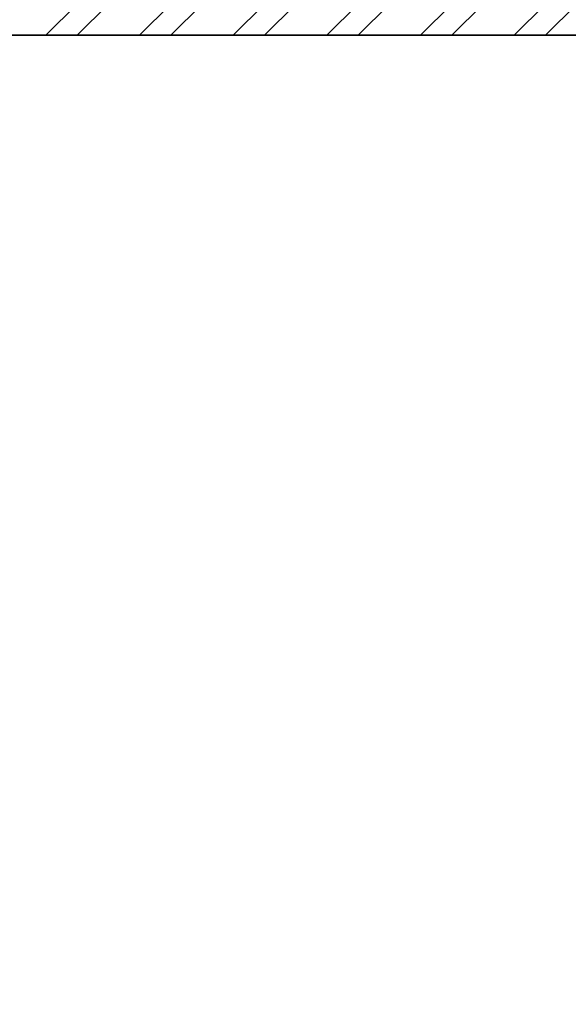
# Model space of a CAD drawing. Units: inches. Extents: x 1885 to 2748, y 783 to 2421.
# Tile 86 of 117: x 2215 to 2294, y 2026 to 2167. Entities that reach past the tile are written whole.
import ezdxf

# ---------------------------------------------------------------- set-up
doc = ezdxf.new("R2010")
doc.units = ezdxf.units.IN
doc.layers.add('A-WALL', color=7, linetype='Continuous', lineweight=35)
doc.layers.add('A-WALL-PATT', color=85, linetype='Continuous', lineweight=13, true_color=0x58ba48)

msp = doc.modelspace()

# ---------------------------------------------------------------- hatches: boundary and pattern name
at = {"layer": 'A-WALL-PATT'}
h = msp.add_hatch(dxfattribs=at)
h.set_pattern_fill('ANSI32', color=256)
h.paths.add_polyline_path([(2007.77, 2318.01), (1980.77, 2318.01), (1980.77, 2281.22), (1985.27, 2281.22), (1985.27, 2313.51), (2007.77, 2313.51), (2007.77, 2315.76)])
h.paths.add_polyline_path([(2094.32, 2318.01), (2067.77, 2318.01), (2067.77, 2313.51), (2094.32, 2313.51), (2094.32, 2315.76)])
h.paths.add_polyline_path([(2131.37, 2315.76), (2131.37, 2318.01), (2131.19, 2318.01), (2112.61, 2318.01), (2112.61, 2313.51), (2117.27, 2313.51), (2117.27, 2255.2), (2121.77, 2255.2), (2121.77, 2313.51), (2131.37, 2313.51)])
h.paths.add_polyline_path([(2190.51, 2318.01), (2155.37, 2318.01), (2155.37, 2313.51), (2169.77, 2313.51), (2169.77, 2229.51), (2121.77, 2229.51), (2121.77, 2233.45), (2119.52, 2233.45), (2117.27, 2233.45), (2117.27, 2201.1), (2121.77, 2201.1), (2121.77, 2225.01), (2169.77, 2225.01), (2169.77, 2165.01), (2306.27, 2165.01), (2306.27, 2066.01), (2310.77, 2066.01), (2344.27, 2066.01), (2486.27, 2066.01), (2486.27, 1886.01), (2483.02, 1886.01), (2483.02, 1881.51), (2486.27, 1881.51), (2486.27, 1880.68), (2490.77, 1880.68), (2490.77, 2070.51), (2344.27, 2070.51), (2310.77, 2070.51), (2310.77, 2165.01), (2310.77, 2173.64), (2308.52, 2173.64), (2306.27, 2173.64), (2306.27, 2169.51), (2174.27, 2169.51), (2174.27, 2313.51), (2190.51, 2313.51), (2190.51, 2315.76)])
h.paths.add_polyline_path([(1985.27, 2221.22), (1980.77, 2221.22), (1980.77, 2165.01), (1992.77, 2165.01), (1992.77, 2141.93), (1997.27, 2141.93), (1997.27, 2165.01), (2117.27, 2165.01), (2117.27, 2163.13), (2121.77, 2163.13), (2121.77, 2172.73), (2119.52, 2172.73), (2117.27, 2172.73), (2117.27, 2169.51), (1985.27, 2169.51)])
h.paths.add_polyline_path([(1997.27, 2105.93), (1992.77, 2105.93), (1992.77, 2070.51), (2016.77, 2070.51), (2016.77, 2059.12), (2019.02, 2059.12), (2021.27, 2059.12), (2021.27, 2070.51), (2117.27, 2070.51), (2117.27, 2022.51), (2114.42, 2022.51), (2114.42, 2018.01), (2123.63, 2018.01), (2123.63, 2020.26), (2123.63, 2022.51), (2121.77, 2022.51), (2121.77, 2142.59), (2119.52, 2142.59), (2117.27, 2142.59), (2117.27, 2075.01), (1997.27, 2075.01)])
h.paths.add_polyline_path([(2092.03, 2020.26), (2092.03, 2022.51), (2021.27, 2022.51), (2021.27, 2035.12), (2016.77, 2035.12), (2016.77, 2018.01), (2016.77, 1978.78), (2021.27, 1978.78), (2021.27, 2018.01), (2092.03, 2018.01)])
h.paths.add_polyline_path([(2260.94, 2022.51), (2153.1, 2022.51), (2153.1, 2020.26), (2153.1, 2018.01), (2155.27, 2018.01), (2155.27, 1886.01), (2107.63, 1886.01), (2107.63, 1881.51), (2182.91, 1881.51), (2182.91, 1883.76), (2182.91, 1886.01), (2159.77, 1886.01), (2159.77, 2018.01), (2260.94, 2018.01), (2260.94, 2020.26)])
h.paths.add_polyline_path([(2047.63, 1883.76), (2047.63, 1886.01), (2021.27, 1886.01), (2021.27, 1918.78), (2019.02, 1918.78), (2016.77, 1918.78), (2016.77, 1881.51), (2047.63, 1881.51)])
h.paths.add_polyline_path([(2306.36, 1883.76), (2306.36, 1886.01), (2296.27, 1886.01), (2296.27, 1982.01), (2316.54, 1982.01), (2316.54, 1984.26), (2316.54, 1986.51), (2296.27, 1986.51), (2296.27, 2022.51), (2289.28, 2022.51), (2289.28, 2018.01), (2291.77, 2018.01), (2291.77, 1886.01), (2242.91, 1886.01), (2242.91, 1881.51), (2306.36, 1881.51)], flags=17)
h.paths.add_polyline_path([(1985.27, 1843.01), (2021.6, 1843.01), (2021.53, 1845.44), (2021.48, 1847.51), (1980.77, 1847.51), (1980.77, 1809.45), (1985.27, 1809.45)])
h.paths.add_polyline_path([(2131.48, 1845.26), (2131.48, 1847.51), (2081.53, 1847.51), (2081.53, 1843.01), (2117.27, 1843.01), (2117.27, 1784.15), (2119.52, 1784.15), (2121.77, 1784.15), (2121.77, 1843.01), (2131.48, 1843.01)])
h.paths.add_polyline_path([(2203.89, 1847.51), (2155.48, 1847.51), (2155.48, 1843.01), (2169.77, 1843.01), (2169.77, 1759.01), (2121.77, 1759.01), (2121.77, 1761.46), (2117.27, 1761.46), (2117.27, 1730.43), (2121.77, 1730.43), (2121.77, 1754.51), (2177.42, 1754.51), (2177.42, 1756.76), (2177.42, 1759.01), (2174.27, 1759.01), (2174.27, 1843.01), (2203.89, 1843.01)])
h.paths.add_polyline_path([(2335.55, 1845.26), (2335.55, 1847.51), (2239.89, 1847.51), (2239.89, 1843.01), (2306.27, 1843.01), (2306.27, 1759.01), (2199.49, 1759.01), (2199.49, 1754.51), (2310.77, 1754.51), (2310.77, 1843.01), (2335.55, 1843.01)])
h.paths.add_polyline_path([(2348.77, 2022.51), (2344.27, 2022.51), (2344.27, 1986.51), (2341.68, 1986.51), (2341.68, 1982.01), (2344.27, 1982.01), (2344.27, 1886.01), (2330.36, 1886.01), (2330.36, 1881.51), (2361.63, 1881.51), (2361.63, 1883.76), (2361.63, 1886.01), (2348.77, 1886.01)], flags=17)
h.paths.add_polyline_path([(2283.25, 2315.76), (2283.25, 2318.01), (2238.51, 2318.01), (2238.51, 2313.51), (2283.25, 2313.51)], flags=17)
h.paths.add_polyline_path([(2363.27, 2348.01), (2388.68, 2348.01), (2388.68, 2350.26), (2388.68, 2352.51), (2358.77, 2352.51), (2358.77, 2348.01), (2358.77, 2318.01), (2344.48, 2318.01), (2344.48, 2313.51), (2358.77, 2313.51), (2358.77, 2229.51), (2310.77, 2229.51), (2310.77, 2231.95), (2306.27, 2231.95), (2306.27, 2205.61), (2310.77, 2205.61), (2310.77, 2225.01), (2358.77, 2225.01), (2358.77, 2211.51), (2452.33, 2211.51), (2452.33, 2213.76), (2452.33, 2216.01), (2363.27, 2216.01), (2363.27, 2318.01)])
h.paths.add_polyline_path([(2310.77, 2313.51), (2320.48, 2313.51), (2320.48, 2315.76), (2320.48, 2318.01), (2302.73, 2318.01), (2302.73, 2313.51), (2306.27, 2313.51), (2306.27, 2251.08), (2310.77, 2251.08)], flags=17)
h.paths.add_polyline_path([(2490.77, 2352.51), (2486.27, 2352.51), (2448.68, 2352.51), (2448.68, 2348.01), (2486.27, 2348.01), (2486.27, 2318.01), (2486.27, 2216.01), (2481.78, 2216.01), (2481.78, 2211.51), (2486.27, 2211.51), (2486.27, 2165.01), (2493.29, 2165.01), (2493.29, 2167.26), (2493.29, 2169.51), (2490.77, 2169.51), (2490.77, 2313.51), (2494.43, 2313.51), (2494.43, 2318.01), (2490.77, 2318.01)])
h.paths.add_polyline_path([(2534.65, 2318.01), (2515.69, 2318.01), (2515.69, 2313.51), (2534.65, 2313.51), (2534.65, 2315.76)])
h.paths.add_polyline_path([(2618.27, 2318.01), (2594.65, 2318.01), (2594.65, 2313.51), (2613.77, 2313.51), (2613.77, 2281.71), (2618.27, 2281.71)])
h.paths.add_polyline_path([(2618.27, 2221.71), (2613.77, 2221.71), (2613.77, 2169.51), (2554.02, 2169.51), (2554.02, 2165.01), (2613.77, 2165.01), (2613.77, 2152.88), (2618.27, 2152.88)])
h.paths.add_polyline_path([(2618.27, 2128.88), (2616.02, 2128.88), (2613.77, 2128.88), (2613.77, 2117.01), (2529.77, 2117.01), (2529.77, 2165.01), (2532.85, 2165.01), (2532.85, 2169.51), (2522.87, 2169.51), (2522.87, 2165.01), (2525.27, 2165.01), (2525.27, 2117.01), (2525.27, 2112.51), (2525.27, 2108.58), (2529.77, 2108.58), (2529.77, 2112.51), (2613.77, 2112.51), (2613.77, 2080.19), (2618.27, 2080.19)])
h.paths.add_polyline_path([(2618.27, 2044.19), (2616.02, 2044.19), (2613.77, 2044.19), (2613.77, 2015.51), (2529.77, 2015.51), (2529.77, 2088.58), (2527.52, 2088.58), (2525.27, 2088.58), (2525.27, 2011.01), (2613.77, 2011.01), (2613.77, 1956.75), (2618.27, 1956.75)])
h.paths.add_polyline_path([(2618.27, 1881.51), (2618.27, 1896.75), (2613.77, 1896.75), (2613.77, 1881.51), (2613.77, 1847.51), (2592.71, 1847.51), (2592.71, 1843.01), (2613.77, 1843.01), (2613.77, 1765.01), (2613.77, 1760.51), (2609.62, 1760.51), (2609.62, 1756.01), (2613.77, 1756.01), (2613.77, 1660.01), (2608.54, 1660.01), (2608.54, 1655.51), (2613.77, 1655.51), (2613.77, 1508.16), (2618.27, 1508.16)])
h.paths.add_polyline_path([(2565.77, 1843.01), (2569, 1843.01), (2569, 1847.51), (2490.77, 1847.51), (2490.77, 1849.7), (2488.52, 1849.7), (2486.27, 1849.7), (2486.27, 1847.51), (2477.27, 1847.51), (2477.27, 1838.51), (2477.27, 1821.49), (2486.27, 1821.49), (2486.27, 1838.51), (2561.27, 1838.51), (2561.27, 1765.01), (2486.27, 1765.01), (2486.27, 1786.16), (2477.27, 1786.16), (2477.27, 1765.01), (2477.27, 1756.01), (2486.27, 1756.01), (2565.77, 1756.01), (2585.62, 1756.01), (2585.62, 1758.26), (2585.62, 1760.51), (2565.77, 1760.51), (2565.77, 1765.01)])
h.paths.add_polyline_path([(2486.27, 1651.01), (2561.27, 1651.01), (2561.27, 1567.01), (2486.27, 1567.01), (2486.27, 1591.32), (2477.27, 1591.32), (2477.27, 1567.01), (2477.27, 1558.01), (2477.27, 1555.44), (2481.77, 1555.44), (2481.77, 1558.01), (2568.65, 1558.01), (2568.65, 1560.26), (2568.65, 1562.51), (2565.77, 1562.51), (2565.77, 1655.51), (2584.54, 1655.51), (2584.54, 1657.76), (2584.54, 1660.01), (2565.77, 1660.01), (2486.27, 1660.01), (2477.27, 1660.01), (2477.27, 1651.01), (2477.27, 1632.99), (2486.27, 1632.99)])
h.paths.add_polyline_path([(2449.97, 1883.76), (2449.97, 1886.01), (2421.63, 1886.01), (2421.63, 1881.51), (2449.97, 1881.51)], flags=17)
h.paths.add_polyline_path([(2447.27, 1847.51), (2395.55, 1847.51), (2395.55, 1843.01), (2442.77, 1843.01), (2442.77, 1809.27), (2447.27, 1809.27)])
h.paths.add_polyline_path([(1985.27, 1749.45), (1980.77, 1749.45), (1980.77, 1694.5), (1985.27, 1694.5), (1985.27, 1694.51), (1986.9, 1694.51), (1986.9, 1697.78), (1986.9, 1699.01), (1985.27, 1699.01)])
h.paths.add_polyline_path([(2152.77, 1699.01), (2121.77, 1699.01), (2121.77, 1703.67), (2119.52, 1703.67), (2117.27, 1703.67), (2117.27, 1699.01), (2009.22, 1699.01), (2009.22, 1694.51), (2148.27, 1694.51), (2148.27, 1692.63), (2152.77, 1692.63)])
h.paths.add_polyline_path([(2016.27, 1694.51), (2011.77, 1694.51), (2011.77, 1558.01), (2040.81, 1558.01), (2040.81, 1560.26), (2040.81, 1562.51), (2016.27, 1562.51)])
h.paths.add_polyline_path([(2152.77, 1663.02), (2150.52, 1663.02), (2148.27, 1663.02), (2148.27, 1562.51), (2100.81, 1562.51), (2100.81, 1558.01), (2165.12, 1558.01), (2165.12, 1560.26), (2165.12, 1562.51), (2152.77, 1562.51), (2152.77, 1610.51), (2224.77, 1610.51), (2224.77, 1607.99), (2229.27, 1607.99), (2229.27, 1615.01), (2152.77, 1615.01)])
h.paths.add_polyline_path([(2238.61, 1560.26), (2238.61, 1562.51), (2229.27, 1562.51), (2229.27, 1588.76), (2227.02, 1588.76), (2224.77, 1588.77), (2224.77, 1562.51), (2189.12, 1562.51), (2189.12, 1558.01), (2238.61, 1558.01)])
h.paths.add_polyline_path([(2336.02, 1560.26), (2336.02, 1562.51), (2310.77, 1562.51), (2310.77, 1656.35), (2308.52, 1656.35), (2306.27, 1656.35), (2306.27, 1562.51), (2286.61, 1562.51), (2286.61, 1558.01), (2336.02, 1558.01)])
h.paths.add_polyline_path([(2447.27, 1690.97), (2445.02, 1690.97), (2442.77, 1690.97), (2442.77, 1687.01), (2306.27, 1687.01), (2306.27, 1680.75), (2310.77, 1680.75), (2310.77, 1682.51), (2442.77, 1682.51), (2442.77, 1562.51), (2396.02, 1562.51), (2396.02, 1558.01), (2447.27, 1558.01)])
h.paths.add_polyline_path([(2447.27, 1749.27), (2445.02, 1749.27), (2442.77, 1749.27), (2442.77, 1717.23), (2447.27, 1717.23)])
h.paths.add_polyline_path([(2044.67, 1521.76), (2044.67, 1524.01), (2007.27, 1524.01), (2007.27, 1503.49), (2009.52, 1503.49), (2011.77, 1503.49), (2011.77, 1519.51), (2044.67, 1519.51)])
h.paths.add_polyline_path([(2177.97, 1521.76), (2177.97, 1524.01), (2104.67, 1524.01), (2104.67, 1519.51), (2145.77, 1519.51), (2145.77, 1387.51), (2143.37, 1387.51), (2143.37, 1383.01), (2251.59, 1383.01), (2251.59, 1385.26), (2251.59, 1387.51), (2150.27, 1387.51), (2150.27, 1519.51), (2177.97, 1519.51)])
h.paths.add_polyline_path([(2298.7, 1524.01), (2237.97, 1524.01), (2237.97, 1519.51), (2282.27, 1519.51), (2282.27, 1387.51), (2279.68, 1387.51), (2279.68, 1383.01), (2286.77, 1383.01), (2286.77, 1419.01), (2312.45, 1419.01), (2312.45, 1421.26), (2312.45, 1423.51), (2286.77, 1423.51), (2286.77, 1519.51), (2298.7, 1519.51), (2298.7, 1521.72)], flags=17)
h.paths.add_polyline_path([(2361.9, 1521.76), (2361.9, 1524.01), (2322.7, 1524.01), (2322.7, 1519.51), (2334.77, 1519.51), (2334.77, 1423.51), (2331.93, 1423.51), (2331.93, 1419.01), (2334.77, 1419.01), (2334.77, 1387.51), (2334.77, 1383.23), (2339.27, 1383.23), (2339.27, 1387.51), (2339.27, 1519.51), (2361.9, 1519.51)], flags=17)
h.paths.add_polyline_path([(2447.27, 1521.76), (2447.27, 1524.01), (2421.9, 1524.01), (2421.9, 1519.51), (2447.27, 1519.51)], flags=17)
h.paths.add_polyline_path([(2481.77, 1529.6), (2479.52, 1529.6), (2477.27, 1529.6), (2477.27, 1524.01), (2474.49, 1524.01), (2474.49, 1519.51), (2477.27, 1519.51), (2477.27, 1334.51), (2296.77, 1334.51), (2296.77, 1240.51), (2160.27, 1240.51), (2160.27, 1180.51), (2112.27, 1180.51), (2112.27, 1207.69), (2110.02, 1207.69), (2107.77, 1207.69), (2107.77, 1171.61), (2112.27, 1171.61), (2112.27, 1176.01), (2160.27, 1176.01), (2160.27, 1092.01), (2144.22, 1092.01), (2144.22, 1087.51), (2189.5, 1087.51), (2189.5, 1089.76), (2189.5, 1092.01), (2164.77, 1092.01), (2164.77, 1236.01), (2296.77, 1236.01), (2296.77, 1231.91), (2301.27, 1231.91), (2301.27, 1330.01), (2481.77, 1330.01), (2481.77, 1387.51)])
h.paths.add_polyline_path([(2618.27, 1448.16), (2613.77, 1448.16), (2613.77, 1382.51), (2529.77, 1382.51), (2525.27, 1382.51), (2525.27, 1307.06), (2529.77, 1307.06), (2529.77, 1378.01), (2613.77, 1378.01), (2613.77, 1354.99), (2618.27, 1354.99)])
h.paths.add_polyline_path([(2618.27, 1318.99), (2613.77, 1318.99), (2613.77, 1281.01), (2529.77, 1281.01), (2529.77, 1283.79), (2527.52, 1283.79), (2525.27, 1283.79), (2525.27, 1228.51), (2516.79, 1228.51), (2516.79, 1224.01), (2533.48, 1224.01), (2533.48, 1226.26), (2533.48, 1228.51), (2529.77, 1228.51), (2529.77, 1276.51), (2613.77, 1276.51), (2613.77, 1266.02), (2618.27, 1266.02)])
h.paths.add_polyline_path([(2618.27, 1134.96), (2613.77, 1134.96), (2613.77, 1092.01), (2594.54, 1092.01), (2594.54, 1087.51), (2618.27, 1087.51)])
h.paths.add_polyline_path([(2534.54, 1092.01), (2509.77, 1092.01), (2509.77, 1087.51), (2534.54, 1087.51), (2534.54, 1089.76)])
h.paths.add_polyline_path([(2481.27, 1224.01), (2484.12, 1224.01), (2484.12, 1226.26), (2484.12, 1228.51), (2476.77, 1228.51), (2476.77, 1198.51), (2471.61, 1198.51), (2471.61, 1194.01), (2476.77, 1194.01), (2476.77, 1062.01), (2436.89, 1062.01), (2436.89, 1057.51), (2476.77, 1057.51), (2481.27, 1057.51), (2481.27, 1062.01), (2481.27, 1087.51), (2485.35, 1087.51), (2485.35, 1089.76), (2485.35, 1092.01), (2481.27, 1092.01), (2481.27, 1117.51)])
h.paths.add_polyline_path([(2439.9, 1198.51), (2349.27, 1198.51), (2349.27, 1194.01), (2349.27, 1180.51), (2301.27, 1180.51), (2301.27, 1201.9), (2299.02, 1201.9), (2296.77, 1201.9), (2296.77, 1172.34), (2299.02, 1172.34), (2301.27, 1172.34), (2301.27, 1176.01), (2349.27, 1176.01), (2349.27, 1092.01), (2334.45, 1092.01), (2334.45, 1087.51), (2349.27, 1087.51), (2349.27, 1057.51), (2353.77, 1057.51), (2376.89, 1057.51), (2376.89, 1059.76), (2376.89, 1062.01), (2353.77, 1062.01), (2353.77, 1087.51), (2353.77, 1180.51), (2353.77, 1194.01), (2439.9, 1194.01), (2439.9, 1196.26)])
h.paths.add_polyline_path([(2270.6, 1089.76), (2270.6, 1092.01), (2249.5, 1092.01), (2249.5, 1087.51), (2270.6, 1087.51)], flags=17)
h.paths.add_polyline_path([(2310.45, 1092.01), (2301.27, 1092.01), (2301.27, 1153.29), (2296.77, 1153.29), (2296.77, 1092.01), (2293.79, 1092.01), (2293.79, 1087.51), (2310.45, 1087.51), (2310.45, 1089.76)], flags=17)
h.paths.add_polyline_path([(2112.27, 1150.33), (2110.02, 1150.33), (2107.77, 1150.33), (2107.77, 1092.01), (2104.47, 1092.01), (2104.47, 1087.51), (2120.22, 1087.51), (2120.22, 1089.76), (2120.22, 1092.01), (2112.27, 1092.01)])
h.paths.add_polyline_path([(2082.17, 1092.01), (2058.14, 1092.01), (2058.14, 1087.51), (2082.17, 1087.51), (2082.17, 1089.76)])
h.paths.add_polyline_path([(1975.77, 1145.64), (1971.27, 1145.64), (1971.27, 1087.51), (1980.77, 1087.51), (1998.14, 1087.51), (1998.14, 1089.76), (1998.14, 1092.01), (1985.27, 1092.01), (1975.77, 1092.01)])
h.paths.add_polyline_path([(2112.27, 1244.38), (2110.02, 1244.38), (2107.77, 1244.38), (2107.77, 1240.51), (1992.27, 1240.51), (1992.27, 1271.01), (1987.77, 1271.01), (1987.77, 1240.51), (1980.77, 1240.51), (1975.77, 1240.51), (1971.27, 1240.51), (1971.27, 1205.64), (1975.77, 1205.64), (1975.77, 1236.01), (2107.77, 1236.01), (2107.77, 1233.44), (2112.27, 1233.44), (2112.27, 1236.01)])
h.paths.add_polyline_path([(2112.27, 1383.01), (2114.78, 1383.01), (2114.78, 1385.26), (2114.78, 1387.51), (2102.48, 1387.51), (2102.48, 1383.01), (2107.77, 1383.01), (2107.77, 1335.01), (2011.77, 1335.01), (2011.77, 1349.94), (2007.27, 1349.94), (2007.27, 1335.01), (1987.77, 1335.01), (1987.77, 1330.51), (1987.77, 1307.01), (1992.27, 1307.01), (1992.27, 1330.51), (2007.27, 1330.51), (2107.77, 1330.51), (2107.77, 1264.71), (2112.27, 1264.71)])
h.paths.add_polyline_path([(2077.86, 1387.51), (2011.77, 1387.51), (2011.77, 1390.04), (2009.52, 1390.04), (2007.27, 1390.04), (2007.27, 1373.94), (2011.77, 1373.94), (2011.77, 1383.01), (2077.86, 1383.01)])
h.paths.add_polyline_path([(2011.77, 1443.49), (2007.27, 1443.49), (2007.27, 1410.25), (2011.77, 1410.25)])

# ---------------------------------------------------------------- linework, layer by layer
at = {"layer": 'A-WALL'}
msp.add_line((2169.77, 2165.01), (2306.27, 2165.01), dxfattribs=at)

doc.saveas('drawing.dxf')
